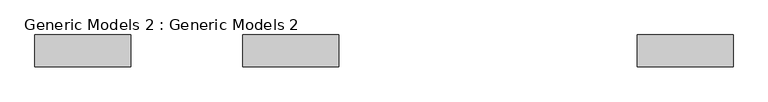
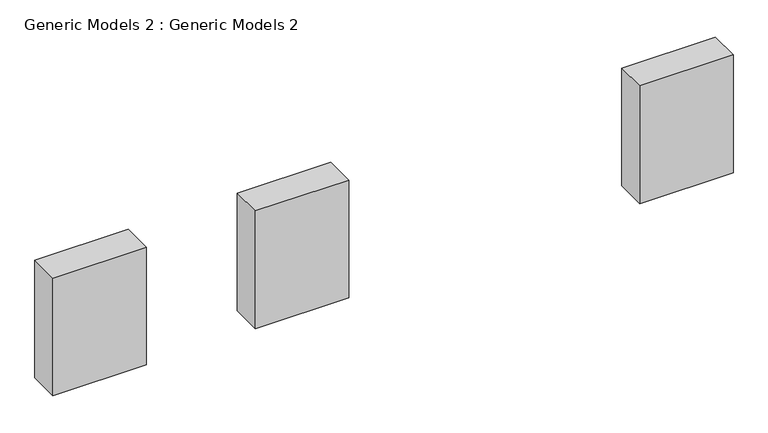
"""IFC4 building model written with IfcOpenShell, lengths in millimetres: proxy geometry, Generic Models 2 : Generic Models 2."""

from ifc_helpers import new_model, si_unit, frame, origin, place, context, project, spatial, polyline, outline, extrude, source, transform, mapped, element, save


def generic_models_2_generic_models_2_5a51ac4f(model_context):
    return source(origin(), model_context, "Body", "SweptSolid", [
        extrude(outline(polyline([(6017.4798531, -8164.8977377), (5103.0798531, -8164.8977377), (5103.0798531, -7860.0977377), (6017.4798531, -7860.0977377), (6017.4798531, -8164.8977377)])), frame((0.0, 0.0, 109.3639159), z_axis=(0.0, 0.0, 1.0), x_axis=(1.0, 0.0, 0.0)), (0.0, 0.0, 1.0), 1219.2),
        extrude(outline(polyline([(2256.2108144, -8164.8977377), (1341.8108144, -8164.8977377), (1341.8108144, -7860.0977377), (2256.2108144, -7860.0977377), (2256.2108144, -8164.8977377)])), frame((0.0, 0.0, 131.9263125), z_axis=(0.0, 0.0, 1.0), x_axis=(1.0, 0.0, 0.0)), (0.0, 0.0, 1.0), 1219.2),
        extrude(outline(polyline([(275.0108144, -8164.8977377), (-639.3891856, -8164.8977377), (-639.3891856, -7860.0977377), (275.0108144, -7860.0977377), (275.0108144, -8164.8977377)])), frame((0.0, 0.0, 131.9263125), z_axis=(0.0, 0.0, 1.0), x_axis=(1.0, 0.0, 0.0)), (0.0, 0.0, 1.0), 1219.2),
    ])


if __name__ == "__main__":
    model = new_model("IFC4")
    model_context = context("Model", 3, world=origin())
    ifc_project = project(units=[si_unit("LENGTHUNIT", "METRE", prefix="MILLI")], contexts=[model_context])
    site = spatial("IfcSite", under=ifc_project)
    building = spatial("IfcBuilding", under=site)
    placement = place(None, origin())
    generic_models_2_generic_models_2_shape = generic_models_2_generic_models_2_5a51ac4f(model_context)
    element("IfcBuildingElementProxy", 1, Name="Generic Models 2 : Generic Models 2", ObjectType="Generic Models 2 : Generic Models 2", at=placement, inside=building, context=model_context, shape_type="MappedRepresentation", body=[
        mapped(generic_models_2_generic_models_2_shape, transform((0.0, 0.0, 0.0), x_axis=(1.0, 0.0, 0.0), y_axis=(0.0, 1.0, 0.0), z_axis=(0.0, 0.0, 1.0))),
    ])
    save(model, "model.ifc")

# Revit data of these elements
# Element 1 (IfcBuildingElementProxy, "Generic Models 2 : Generic Models 2")
#   Materials on its faces: "Parking Stripe"
# Materials
#   "Parking Stripe": class "Paint", colour RGB 250 250 91, transparency 0, Cost = 0
